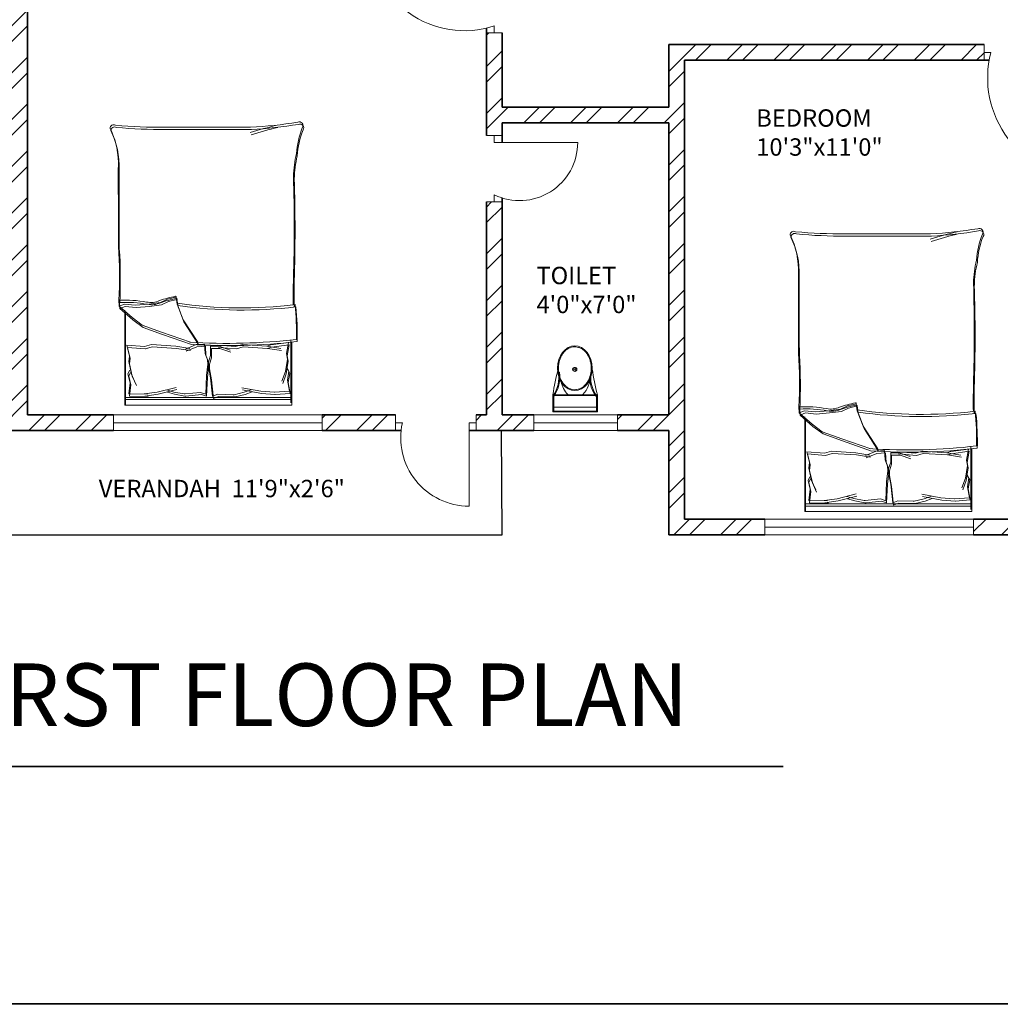
# Model space of a CAD drawing. Units: inches. Extents: x 1885 to 2748, y 783 to 2421.
# Tile 21 of 117: x 2163 to 2445, y 922 to 1206. Entities that reach past the tile are written whole.
import ezdxf

# ---------------------------------------------------------------- set-up
doc = ezdxf.new("R2010")
doc.units = ezdxf.units.IN
for name, color, linetype, lineweight in [('A-ANNO-DIMS', 2, 'Continuous', 18), ('A-ANNO-TTLB', 7, 'Continuous', 35), ('A-AREA-IDEN', 7, 'Continuous', 18), ('A-DOOR', 31, 'Continuous', 18), ('A-FLOR-BALC', 7, 'Continuous', 25), ('A-FLOR-FIXT', 8, 'Continuous', 18), ('A-FURN', 8, 'Continuous', 13), ('A-GLAZ', 181, 'Continuous', 18), ('A-WALL', 7, 'Continuous', 35)]:
    doc.layers.add(name, color=color, linetype=linetype, lineweight=lineweight)
doc.layers.add('A-WALL-PATT', color=85, linetype='Continuous', lineweight=13, true_color=0x58ba48)
doc.styles.get("Standard").update_dxf_attribs({"font": 'arial.ttf'})
doc.dimstyles.get("Standard").update_dxf_attribs({"dimtxt": 0.18, "dimasz": 0.18, "dimexe": 0.18, "dimexo": 0.0625, "dimgap": 0.09, "dimtad": 0, "dimtih": 1, "dimtoh": 1, "dimdec": 4, "dimzin": 0, "dimdsep": 46, "dimtxsty": 'Standard', "dimcen": 0.09, "dimadec": 0, "dimazin": 0, "dimtfac": 1, "dimtdec": 4, "dimtofl": 0, "dimtmove": 0, "dimatfit": 3, "dimfxl": 1, "dimtolj": 1, "dimtzin": 0, "dimarcsym": 0})

# ---------------------------------------------------------------- blocks, each defined once
blk = doc.blocks.new('A$C31115884')
for p, q in [((283, 498), (223, 498)), ((258, 466), (258, 523)), ((0, 200), (0, 0)), ((520, 200), (0, 200)), ((10, 190), (10, 10)), ((510, 190), (10, 190)), ((510, 10), (510, 190)), ((520, 0), (520, 200)), ((510, 54), (0, 54)), ((10, 10), (510, 10)), ((0, 0), (520, 0))]:
    blk.add_line(p, q)
blk.add_circle((256, 496), 23.6)
for centre, radius, start, end in [((2778, -205), 2807, 165.4549, 171.7133), ((-295, 403), 365, 324.2091, 9.3499), ((-295, 403), 375, 324.2091, 9.3499), ((806, 403), 365, 170.6501, 215.7909), ((3237, 905), 2807, 188.2867, 194.5451), ((384, 406), 293, 190.2774, 224.1564), ((139, 406), 293, 315.8436, 2.6563), ((806, 403), 375, 179.2036, 215.7909)]:
    blk.add_arc(centre, radius, start, end)
blk.add_ellipse((256, 510), major_axis=(0, -261), ratio=0.772727)
blk.add_open_spline([(256, 259), (263, 259), (270, 260), (288, 262), (299, 265), (320, 273), (330, 278), (350, 291), (360, 299), (378, 316), (386, 326), (402, 347), (409, 358), (421, 383), (427, 395), (436, 422), (440, 436), (445, 465), (447, 480), (448, 509), (448, 524), (445, 553), (443, 568), (436, 596), (432, 610), (422, 636), (416, 649), (402, 672), (395, 683), (379, 703), (370, 712), (351, 728), (341, 735), (321, 746), (310, 751), (289, 757), (278, 759), (256, 761), (245, 761), (223, 757), (212, 754), (191, 746), (181, 741), (161, 728), (151, 720), (133, 703), (125, 693), (110, 672), (103, 660), (90, 636), (85, 623), (76, 596), (72, 582), (67, 553), (66, 538), (64, 509), (65, 494), (68, 465), (70, 450), (77, 422), (81, 408), (91, 382), (97, 370), (111, 346), (118, 335), (135, 316), (144, 307), (162, 291), (172, 284), (193, 273), (203, 269), (225, 262), (236, 260), (250, 259), (253, 259), (256, 259)], degree=3, knots=[0, 0, 0, 0, 0.110105, 0.110105, 0.285049, 0.285049, 0.459994, 0.459994, 0.634938, 0.634938, 0.809882, 0.809882, 0.984827, 0.984827, 1.159771, 1.159771, 1.334715, 1.334715, 1.50966, 1.50966, 1.684604, 1.684604, 1.859549, 1.859549, 2.034493, 2.034493, 2.209437, 2.209437, 2.384382, 2.384382, 2.559326, 2.559326, 2.73427, 2.73427, 2.909215, 2.909215, 3.084159, 3.084159, 3.259103, 3.259103, 3.434048, 3.434048, 3.608992, 3.608992, 3.783936, 3.783936, 3.958881, 3.958881, 4.133825, 4.133825, 4.30877, 4.30877, 4.483714, 4.483714, 4.658658, 4.658658, 4.833603, 4.833603, 5.008547, 5.008547, 5.183491, 5.183491, 5.358436, 5.358436, 5.53338, 5.53338, 5.708324, 5.708324, 5.883269, 5.883269, 6.058213, 6.058213, 6.233158, 6.233158, 6.283185, 6.283185, 6.283185, 6.283185])
blk = doc.blocks.new('BED-DOUBLE')
for p, q in [((0, 51.49), (0.64, 51.49)), ((0, 3.47), (0, 51.49)), ((0, 51.26), (26.61, 51.26)), ((0, 51.26), (26.61, 51.26)), ((0.64, 51.49), (27.25, 51.49)), ((0.64, 51.49), (27.25, 51.49)), ((1.54, 3.47), (1.54, 51.26)), ((1.54, 3.47), (1.54, 51.26)), ((2.18, 3.7), (2.18, 51.49)), ((2.18, 3.7), (2.18, 51.49)), ((27.75, 52.87), (24.5, 49.16)), ((27.75, 52.87), (24.5, 49.16)), ((28.39, 53.09), (25.14, 49.39)), ((28.39, 53.09), (25.14, 49.39)), ((29.49, 52.95), (27.75, 52.87, 3.87)), ((29.49, 52.95), (27.75, 52.87, 3.87)), ((28.37, 51.33), (27.75, 52.87)), ((28.37, 51.33), (27.75, 52.87)), ((28.06, 48.23), (28.37, 51.33)), ((28.06, 48.23), (28.37, 51.33)), ((30.13, 53.17), (28.39, 53.09, 3.87)), ((30.13, 53.17), (28.39, 53.09, 3.87)), ((29.01, 51.56), (28.39, 53.09)), ((29.01, 51.56), (28.39, 53.09)), ((28.7, 48.46), (29.01, 51.56)), ((28.7, 48.46), (29.01, 51.56)), ((2.56, 50.11), (2.46, 44.71)), ((2.56, 50.11), (2.46, 44.71)), ((2.56, 50.11), (5.77, 49.73)), ((2.56, 50.11), (5.77, 49.73)), ((3.2, 50.34), (3.1, 44.94)), ((3.2, 50.34), (3.1, 44.94)), ((3.2, 50.34), (6.41, 49.96)), ((3.2, 50.34), (6.41, 49.96)), ((8.26, 49.31), (5.58, 48.13)), ((8.26, 49.31), (5.58, 48.13)), ((5.77, 49.73), (8.34, 50.33)), ((5.77, 49.73), (8.34, 50.33)), ((8.9, 49.54), (6.22, 48.36)), ((8.9, 49.54), (6.22, 48.36)), ((6.41, 49.96), (8.98, 50.56)), ((6.41, 49.96), (8.98, 50.56)), ((11.83, 50.11), (8.26, 49.31)), ((11.83, 50.11), (8.26, 49.31)), ((8.34, 50.33), (9.39, 49.81)), ((8.34, 50.33), (9.39, 49.81)), ((12.47, 50.34), (8.9, 49.54)), ((12.47, 50.34), (8.9, 49.54)), ((8.98, 50.56), (10.03, 50.04)), ((8.98, 50.56), (10.03, 50.04)), ((13.44, 49.92), (11.83, 50.11)), ((13.44, 49.92), (11.83, 50.11)), ((14.08, 50.15), (12.47, 50.34)), ((14.08, 50.15), (12.47, 50.34)), ((16.58, 50.7), (13.44, 49.92)), ((16.58, 50.7), (13.44, 49.92)), ((17.22, 50.93), (14.08, 50.15)), ((17.22, 50.93), (14.08, 50.15)), ((16.17, 45.57), (16.58, 50.7)), ((16.17, 45.56), (16.58, 50.7)), ((16.81, 45.79), (17.22, 50.93)), ((16.81, 45.79), (17.22, 50.93)), ((24.5, 49.16), (22.33, 46.22)), ((24.5, 49.16), (22.33, 46.22)), ((25.14, 49.39), (22.97, 46.45)), ((25.14, 49.39), (22.97, 46.45)), ((28.37, 44.36), (28.06, 48.23)), ((28.37, 44.36), (28.06, 48.23)), ((29.01, 44.59), (28.7, 48.46)), ((29.01, 44.59), (28.7, 48.46)), ((2.46, 44.71), (2.55, 45.71)), ((2.46, 44.71), (2.55, 45.71)), ((2.55, 45.71), (3.07, 41.91)), ((2.55, 45.71), (3.07, 41.91)), ((3.1, 44.94), (3.19, 45.94)), ((3.1, 44.94), (3.19, 45.94)), ((3.19, 45.94), (3.71, 42.14)), ((3.19, 45.94), (3.71, 42.14)), ((16.73, 43.6), (16.17, 45.57)), ((16.73, 43.6), (16.17, 45.56)), ((17.37, 43.83), (16.81, 45.79)), ((17.37, 43.83), (16.81, 45.79)), ((22.33, 46.22), (20.32, 40.64)), ((22.33, 46.22), (20.32, 40.64)), ((22.97, 46.45), (20.96, 40.87)), ((22.97, 46.45), (20.96, 40.87)), ((16.3, 36.59), (16.73, 43.6)), ((16.3, 36.59), (16.73, 43.6)), ((16.94, 36.82), (17.37, 43.83)), ((16.94, 36.82), (17.37, 43.83)), ((28.83, 40.95), (28.37, 44.36)), ((28.83, 40.95), (28.37, 44.36)), ((29.47, 41.18), (29.01, 44.59)), ((29.47, 41.18), (29.01, 44.59)), ((3.07, 41.91), (4.43, 36.49)), ((3.07, 41.91), (4.43, 36.49)), ((3.71, 42.14), (5.07, 36.72)), ((3.71, 42.14), (5.07, 36.72)), ((20.32, 40.64), (17.39, 32.3)), ((20.32, 40.64), (17.39, 32.3)), ((20.96, 40.87), (18.03, 32.53)), ((20.96, 40.87), (18.03, 32.53)), ((29.76, 38.94), (28.83, 40.95)), ((29.76, 38.94), (28.83, 40.95)), ((30.4, 39.17), (29.47, 41.18)), ((30.4, 39.17), (29.47, 41.18)), ((79.25, 15.06), (79.25, 39.68)), ((79.25, 15.06), (79.25, 39.68)), ((79.89, 15.29), (79.89, 39.9)), ((79.89, 15.29), (79.89, 39.9)), ((3.08, 37.13), (2.54, 34.2)), ((3.08, 37.13), (2.54, 34.2)), ((3.68, 39.2), (3.08, 37.13)), ((3.68, 39.2), (3.08, 37.13)), ((3.72, 37.36), (3.18, 34.43)), ((3.72, 37.36), (3.18, 34.43)), ((4.32, 39.43), (3.72, 37.36)), ((4.32, 39.43), (3.72, 37.36)), ((16.27, 32.79), (16.94, 36.82)), ((16.27, 32.79), (16.94, 36.82)), ((30.38, 36.46), (29.76, 38.94)), ((30.38, 36.46), (29.76, 38.94)), ((31.02, 36.69), (30.4, 39.17)), ((31.02, 36.69), (30.4, 39.17)), ((2.54, 34.2), (2.56, 33.88)), ((2.54, 34.2), (2.56, 33.88)), ((3.18, 34.43), (3.2, 34.11)), ((3.18, 34.43), (3.2, 34.11)), ((3.2, 34.11), (3.62, 29.68)), ((3.2, 34.11), (3.62, 29.68)), ((15.63, 32.56), (16.3, 36.59)), ((15.63, 32.56), (16.3, 36.59)), ((17.38, 30.98), (16.1, 34.05)), ((17.38, 30.98), (16.1, 34.05)), ((17.39, 30.26), (23.88, 34.45)), ((17.39, 30.26), (23.88, 34.45)), ((18.03, 30.49), (24.52, 34.68)), ((18.03, 30.49), (24.52, 34.68)), ((23.88, 34.45), (28.37, 36.15)), ((23.88, 34.45), (28.37, 36.15)), ((24.52, 34.68), (29.01, 36.38)), ((24.52, 34.68), (29.01, 36.38)), ((28.37, 36.15), (30.38, 36.46)), ((28.37, 36.15), (30.38, 36.46)), ((29.01, 36.38), (31.02, 36.69)), ((29.01, 36.38), (31.02, 36.69)), ((2.56, 33.88), (2.98, 29.45)), ((2.56, 33.88), (2.98, 29.45)), ((16.74, 30.75), (15.46, 33.82)), ((16.74, 30.75), (15.46, 33.82)), ((2.98, 29.45), (2.5, 27.98)), ((2.98, 29.45), (2.5, 27.98)), ((3.62, 29.68), (3.13, 28.2)), ((3.62, 29.68), (3.13, 28.2)), ((13.02, 27.66), (14.86, 28.36)), ((13.02, 27.66), (14.86, 28.36)), ((14.86, 28.36), (17.54, 28.52)), ((14.86, 28.36), (17.54, 28.52)), ((16.9, 28.3), (16.74, 30.75)), ((16.9, 28.3), (16.74, 30.75)), ((17.54, 28.52), (17.38, 30.98)), ((17.54, 28.52), (17.38, 30.98)), ((1.87, 25.98), (7.22, 26.56)), ((1.87, 25.98), (7.22, 26.56)), ((2.45, 24.54), (1.87, 25.98)), ((2.45, 24.54), (1.87, 25.98)), ((2.5, 27.98), (7.87, 27.73)), ((2.5, 27.98), (7.87, 27.73)), ((2.51, 26.21), (7.86, 26.79)), ((2.51, 26.21), (7.86, 26.79)), ((3.09, 24.76), (2.51, 26.21)), ((3.09, 24.76), (2.51, 26.21)), ((3.13, 28.2), (8.51, 27.96)), ((3.13, 28.2), (8.51, 27.96)), ((7.22, 26.56), (10.4, 27.14)), ((7.22, 26.56), (10.4, 27.14)), ((7.86, 26.79), (11.04, 27.37)), ((7.86, 26.79), (11.04, 27.37)), ((7.87, 27.73), (11.08, 27.35)), ((7.87, 27.73), (11.08, 27.35)), ((8.51, 27.96), (11.72, 27.58)), ((8.51, 27.96), (11.72, 27.58)), ((10.4, 27.14), (11.71, 27.14)), ((10.4, 27.14), (11.71, 27.14)), ((11.04, 27.37), (12.35, 27.37)), ((11.04, 27.37), (12.35, 27.37)), ((11.08, 27.35), (12.38, 27.43)), ((11.08, 27.35), (12.38, 27.43)), ((11.71, 27.14), (13.59, 26.56)), ((11.71, 27.14), (13.59, 26.56)), ((11.72, 27.58), (13.02, 27.66)), ((11.72, 27.58), (13.02, 27.66)), ((12.35, 27.37), (14.22, 26.79)), ((12.35, 27.37), (14.22, 26.79)), ((12.38, 27.43), (14.22, 28.13)), ((12.38, 27.43), (14.22, 28.13)), ((13.59, 26.56), (16.27, 26.56)), ((13.59, 26.56), (16.27, 26.56)), ((14.22, 28.13), (16.9, 28.3)), ((14.22, 28.13), (16.9, 28.3)), ((14.22, 26.79), (16.91, 26.79)), ((14.22, 26.79), (16.91, 26.79)), ((16.27, 26.56), (16.27, 24.1)), ((16.27, 26.56), (16.27, 24.1)), ((16.91, 26.79), (16.91, 24.33)), ((16.91, 26.79), (16.91, 24.33)), ((2.31, 20.09), (2.45, 24.54)), ((2.31, 20.09), (2.45, 24.54)), ((2.95, 20.32), (3.09, 24.76)), ((2.95, 20.32), (3.09, 24.76)), ((16.27, 24.1), (15.18, 20.96)), ((16.27, 24.1), (15.18, 20.96)), ((16.91, 24.33), (15.82, 21.19)), ((16.91, 24.33), (15.82, 21.19)), ((16.17, 19.38), (16.58, 24.51)), ((16.17, 19.38), (16.58, 24.51)), ((16.81, 19.61), (17.22, 24.74)), ((16.81, 19.61), (17.22, 24.74)), ((2.31, 19.77), (2.31, 20.09)), ((2.31, 19.77), (2.31, 20.09)), ((2.95, 20), (2.95, 20.32)), ((2.95, 20), (2.95, 20.32)), ((3.67, 17.11), (2.95, 20)), ((3.67, 17.11), (2.95, 20)), ((3.03, 16.88), (2.31, 19.77)), ((3.03, 16.88), (2.31, 19.77)), ((3.32, 12.11), (4.33, 17.6)), ((3.32, 12.11), (4.33, 17.6)), ((4.39, 15.08), (3.67, 17.11)), ((4.39, 15.08), (3.67, 17.11)), ((3.96, 12.34), (4.97, 17.83)), ((3.96, 12.34), (4.97, 17.83)), ((16.73, 17.42), (16.17, 19.38)), ((16.73, 17.42), (16.17, 19.38)), ((16.3, 10.41), (16.73, 17.42)), ((16.3, 10.41), (16.73, 17.42)), ((17.37, 17.65), (16.81, 19.61)), ((17.37, 17.65), (16.81, 19.61)), ((16.94, 10.64), (17.37, 17.65)), ((16.94, 10.64), (17.37, 17.65)), ((3.75, 14.85), (3.03, 16.88)), ((3.75, 14.85), (3.03, 16.88)), ((3.03, 8.28), (3.32, 12.11)), ((3.03, 8.28), (3.32, 12.11)), ((3.67, 8.51), (3.96, 12.34)), ((3.67, 8.51), (3.96, 12.34)), ((3.65, 8.41), (3.67, 8.51)), ((3.65, 8.41), (3.67, 8.51)), ((15.63, 6.38), (16.3, 10.41)), ((15.63, 6.38), (16.3, 10.41)), ((16.27, 6.61), (16.94, 10.64)), ((16.27, 6.61), (16.94, 10.64)), ((16.3, 10.41), (16.62, 9.28)), ((16.3, 10.41), (16.62, 9.28)), ((16.62, 9.28), (17.34, 4.18)), ((16.62, 9.28), (17.34, 4.18)), ((16.94, 10.64), (17.26, 9.51)), ((16.94, 10.64), (17.26, 9.51)), ((17.26, 9.51), (17.98, 4.41)), ((17.26, 9.51), (17.98, 4.41)), ((3.01, 8.18), (3.03, 8.28)), ((3.01, 8.18), (3.03, 8.28)), ((3.34, 3.9), (3.01, 8.18)), ((3.34, 3.9), (3.01, 8.18)), ((3.98, 4.13), (3.65, 8.41)), ((3.98, 4.13), (3.65, 8.41)), ((8.96, 5.05), (6.21, 6.06)), ((8.96, 5.05), (6.21, 6.06)), ((9.6, 5.28), (6.85, 6.29)), ((9.6, 5.28), (6.85, 6.29)), ((18.11, 3.47), (0, 3.47)), ((18.11, 3.47), (0, 3.47)), ((18.75, 3.7), (0.64, 3.7)), ((18.75, 3.7), (0.64, 3.7)), ((3.32, 3.89), (6.5, 4.47)), ((3.32, 3.89), (6.5, 4.47)), ((3.96, 4.12), (7.14, 4.7)), ((3.96, 4.12), (7.14, 4.7)), ((6.5, 4.47), (9.1, 4.04)), ((6.5, 4.47), (9.1, 4.04)), ((7.14, 4.7), (9.74, 4.27)), ((7.14, 4.7), (9.74, 4.27)), ((12.57, 4.47), (8.96, 5.05)), ((12.57, 4.47), (8.96, 5.05)), ((9.1, 4.04), (10.12, 4.62)), ((9.1, 4.04), (10.12, 4.62)), ((13.21, 4.7), (9.6, 5.28)), ((13.21, 4.7), (9.6, 5.28)), ((9.74, 4.27), (10.75, 4.84)), ((9.74, 4.27), (10.75, 4.84)), ((14.16, 4.76), (12.57, 4.47)), ((14.16, 4.76), (12.57, 4.47)), ((14.8, 4.99), (13.21, 4.7)), ((14.8, 4.99), (13.21, 4.7)), ((17.34, 4.18), (14.16, 4.76)), ((17.34, 4.18), (14.16, 4.76)), ((17.98, 4.41), (14.8, 4.99)), ((17.98, 4.41), (14.8, 4.99))]:
    blk.add_line(p, q)
for centre, radius, start, end in [((68.67, 76.16), 23.07, 267.4714, 296.4681), ((68.67, 76.16), 23.07, 267.4714, 296.4681), ((69.31, 76.38), 23.07, 267.4714, 296.4681), ((69.31, 76.38), 23.07, 267.4714, 296.4681), ((78.87, 54.41), 1.1, 332.6588, 86.02), ((78.87, 54.41), 1.1, 332.6588, 86.02), ((212.28, 41.15), 133.04, 174.4998, 180.6351), ((212.28, 41.15), 133.04, 174.4998, 180.6351), ((79.51, 54.64), 1.1, 332.6588, 86.02), ((79.51, 54.64), 1.1, 332.6588, 86.02), ((212.92, 41.38), 133.04, 174.4998, 180.6351), ((212.92, 41.38), 133.04, 174.4998, 180.6351), ((-6.65, 51.33), 36.18, 349.8763, 2.5657), ((-6.65, 51.33), 36.18, 349.8763, 2.5657), ((36.32, 182.26), 129.5, 266.9791, 273.8365), ((36.32, 182.26), 129.5, 266.9791, 273.8365), ((-6.01, 51.55), 36.18, 349.8763, 2.5657), ((-6.01, 51.55), 36.18, 349.8763, 2.5657), ((36.96, 182.49), 129.5, 266.9791, 273.8365), ((36.96, 182.49), 129.5, 266.9791, 273.8365), ((67.83, -4508.74), 4561.86, 90.00217, 90.28689), ((67.83, -4508.75), 4561.86, 90.00217, 90.28689), ((68.46, -4508.52), 4561.86, 90.00217, 90.28689), ((68.46, -4508.52), 4561.86, 90.00217, 90.28689), ((35.07, 43.74), 6.22, 168.6608, 203.7384), ((35.07, 43.74), 6.22, 168.6608, 203.7384), ((35.71, 43.97), 6.22, 168.6608, 203.7384), ((35.71, 43.97), 6.22, 168.6608, 203.7384), ((1.49, 31.15), 29.65, 10.6617, 19.8806), ((1.49, 31.15), 29.65, 10.6617, 19.8806), ((2.13, 31.38), 29.65, 10.6617, 19.8806), ((2.13, 31.38), 29.65, 10.6617, 19.8806), ((31.08, 36.86), 0.185, 250.2464, 1.1377), ((31.08, 36.86), 0.185, 250.2464, 1.1377), ((156.32, 17.75), 129.02, 171.7845, 186.9006), ((156.32, 17.75), 129.02, 171.7845, 186.9006), ((156.96, 17.98), 129.02, 171.7845, 186.9006), ((156.96, 17.98), 129.02, 171.7845, 186.9006), ((30.44, 36.64), 0.185, 250.2464, 1.1377), ((30.44, 36.63), 0.185, 250.2464, 1.1377), ((182.06, 21.36), 164.97, 176.0865, 186.7821), ((182.06, 21.36), 164.97, 176.0865, 186.7821), ((182.7, 21.59), 164.97, 176.0865, 186.7821), ((182.7, 21.59), 164.97, 176.0865, 186.7821), ((-23.71, -17.22), 106.46, 13.3832, 17.7053), ((-23.71, -17.22), 106.46, 13.3832, 17.7053), ((-23.07, -16.99), 106.46, 13.3832, 17.7053), ((-23.07, -16.99), 106.46, 13.3832, 17.7053), ((200.84, 21.43), 121.76, 182.9958, 189.4091), ((200.84, 21.43), 121.76, 182.9958, 189.4091), ((201.48, 21.65), 121.76, 182.9958, 189.4091), ((201.48, 21.65), 121.76, 182.9958, 189.4091), ((31.82, -167.08), 170.11, 88.4762, 91.0082), ((31.82, -167.08), 170.11, 88.4762, 91.0082), ((51.26, 485.05), 482.31, 268.2277, 271.7185), ((51.26, 485.05), 482.31, 268.2277, 271.7185), ((65.16, -26.67), 29.63, 76.0648, 88.9113), ((65.16, -26.67), 29.63, 76.0648, 88.9113), ((20.1, 85.16), 83.31, 268.7218, 275.604), ((20.1, 85.16), 83.31, 268.7218, 275.604), ((20.74, 85.39), 83.31, 268.7218, 275.604), ((20.74, 85.39), 83.31, 268.7218, 275.604), ((31.18, -167.31), 170.11, 88.4762, 91.0082), ((31.18, -167.31), 170.11, 88.4762, 91.0082), ((50.62, 484.82), 482.31, 268.2277, 271.7185), ((50.62, 484.82), 482.31, 268.2277, 271.7185), ((64.52, -26.9), 29.63, 76.0648, 88.9113), ((64.52, -26.9), 29.63, 76.0648, 88.9113), ((70.28, -21.66), 23.56, 67.9751, 86.652), ((70.28, -21.66), 23.56, 67.9751, 86.652), ((70.92, -21.43), 23.56, 67.9751, 86.652), ((70.92, -21.43), 23.56, 67.9751, 86.652), ((79.72, 1.09), 1.09, 236.1736, 23.4781), ((79.72, 1.09), 1.09, 236.1736, 23.4781), ((80.36, 1.31), 1.09, 236.1736, 23.4781), ((80.36, 1.31), 1.09, 236.1736, 23.4781)]:
    blk.add_arc(centre, radius, start, end)
blk = doc.blocks.new('WIN-60')
for p, q in [((0, 60), (4.5, 60)), ((0, 60), (0, 0)), ((4.5, 60), (2.25, 60)), ((2.25, 60), (2.25, 0)), ((4.5, 0), (4.5, 60)), ((2.25, 0), (0, 0)), ((0, 0), (4.5, 0))]:
    blk.add_line(p, q)
blk = doc.blocks.new('WIN-24')
for p, q in [((0, 4.5), (0, 0)), ((0, 4.5), (24, 4.5)), ((24, 2.25), (24, 4.5)), ((24, 4.5), (24, 0)), ((0, 0), (0, 2.25)), ((0, 2.25), (24, 2.25)), ((24, 0), (0, 0))]:
    blk.add_line(p, q)
blk = doc.blocks.new('*D43')
at = {"layer": 'A-ANNO-DIMS', "color": 0, "lineweight": -2, "transparency": 16777216}
for p, q in [((1971.27, 1057.44), (1971.27, 922.48)), ((2618.27, 1057.44), (2618.27, 922.48)), ((1971.45, 922.66), (2294.48, 922.66)), ((2618.09, 922.66), (2295.06, 922.66))]:
    blk.add_line(p, q, dxfattribs=at)
at = {"layer": 'A-ANNO-DIMS', "color": 0, "transparency": 16777216}
for points in [[(1971.45, 922.69), (1971.45, 922.63), (1971.27, 922.66)], [(2618.09, 922.69), (2618.09, 922.63), (2618.27, 922.66)]]:
    blk.add_solid(points, dxfattribs=at)
at = {"layer": 'Defpoints', "color": 0, "transparency": 16777216}
for p in [(1971.27, 1057.51), (2618.27, 1057.51), (2618.27, 922.66)]:
    blk.add_point(p, dxfattribs=at)
at = {"layer": 'A-ANNO-DIMS', "color": 0, "transparency": 16777216, "insert": (2294.77, 922.66), "char_height": 0.18, "attachment_point": 5}
blk.add_mtext('\\A1;647', dxfattribs=at)

msp = doc.modelspace()

# ---------------------------------------------------------------- hatches: boundary and pattern name
at = {"layer": 'A-WALL-PATT'}
h = msp.add_hatch(dxfattribs=at)
h.set_pattern_fill('ANSI32', color=256)
h.paths.add_polyline_path([(2007.77, 2318.01), (1980.77, 2318.01), (1980.77, 2281.22), (1985.27, 2281.22), (1985.27, 2313.51), (2007.77, 2313.51), (2007.77, 2315.76)])
h.paths.add_polyline_path([(2094.32, 2318.01), (2067.77, 2318.01), (2067.77, 2313.51), (2094.32, 2313.51), (2094.32, 2315.76)])
h.paths.add_polyline_path([(2131.37, 2315.76), (2131.37, 2318.01), (2131.19, 2318.01), (2112.61, 2318.01), (2112.61, 2313.51), (2117.27, 2313.51), (2117.27, 2255.2), (2121.77, 2255.2), (2121.77, 2313.51), (2131.37, 2313.51)])
h.paths.add_polyline_path([(2190.51, 2318.01), (2155.37, 2318.01), (2155.37, 2313.51), (2169.77, 2313.51), (2169.77, 2229.51), (2121.77, 2229.51), (2121.77, 2233.45), (2119.52, 2233.45), (2117.27, 2233.45), (2117.27, 2201.1), (2121.77, 2201.1), (2121.77, 2225.01), (2169.77, 2225.01), (2169.77, 2165.01), (2306.27, 2165.01), (2306.27, 2066.01), (2310.77, 2066.01), (2344.27, 2066.01), (2486.27, 2066.01), (2486.27, 1886.01), (2483.02, 1886.01), (2483.02, 1881.51), (2486.27, 1881.51), (2486.27, 1880.68), (2490.77, 1880.68), (2490.77, 2070.51), (2344.27, 2070.51), (2310.77, 2070.51), (2310.77, 2165.01), (2310.77, 2173.64), (2308.52, 2173.64), (2306.27, 2173.64), (2306.27, 2169.51), (2174.27, 2169.51), (2174.27, 2313.51), (2190.51, 2313.51), (2190.51, 2315.76)])
h.paths.add_polyline_path([(1985.27, 2221.22), (1980.77, 2221.22), (1980.77, 2165.01), (1992.77, 2165.01), (1992.77, 2141.93), (1997.27, 2141.93), (1997.27, 2165.01), (2117.27, 2165.01), (2117.27, 2163.13), (2121.77, 2163.13), (2121.77, 2172.73), (2119.52, 2172.73), (2117.27, 2172.73), (2117.27, 2169.51), (1985.27, 2169.51)])
h.paths.add_polyline_path([(1997.27, 2105.93), (1992.77, 2105.93), (1992.77, 2070.51), (2016.77, 2070.51), (2016.77, 2059.12), (2019.02, 2059.12), (2021.27, 2059.12), (2021.27, 2070.51), (2117.27, 2070.51), (2117.27, 2022.51), (2114.42, 2022.51), (2114.42, 2018.01), (2123.63, 2018.01), (2123.63, 2020.26), (2123.63, 2022.51), (2121.77, 2022.51), (2121.77, 2142.59), (2119.52, 2142.59), (2117.27, 2142.59), (2117.27, 2075.01), (1997.27, 2075.01)])
h.paths.add_polyline_path([(2092.03, 2020.26), (2092.03, 2022.51), (2021.27, 2022.51), (2021.27, 2035.12), (2016.77, 2035.12), (2016.77, 2018.01), (2016.77, 1978.78), (2021.27, 1978.78), (2021.27, 2018.01), (2092.03, 2018.01)])
h.paths.add_polyline_path([(2260.94, 2022.51), (2153.1, 2022.51), (2153.1, 2020.26), (2153.1, 2018.01), (2155.27, 2018.01), (2155.27, 1886.01), (2107.63, 1886.01), (2107.63, 1881.51), (2182.91, 1881.51), (2182.91, 1883.76), (2182.91, 1886.01), (2159.77, 1886.01), (2159.77, 2018.01), (2260.94, 2018.01), (2260.94, 2020.26)])
h.paths.add_polyline_path([(2047.63, 1883.76), (2047.63, 1886.01), (2021.27, 1886.01), (2021.27, 1918.78), (2019.02, 1918.78), (2016.77, 1918.78), (2016.77, 1881.51), (2047.63, 1881.51)])
h.paths.add_polyline_path([(2306.36, 1883.76), (2306.36, 1886.01), (2296.27, 1886.01), (2296.27, 1982.01), (2316.54, 1982.01), (2316.54, 1984.26), (2316.54, 1986.51), (2296.27, 1986.51), (2296.27, 2022.51), (2289.28, 2022.51), (2289.28, 2018.01), (2291.77, 2018.01), (2291.77, 1886.01), (2242.91, 1886.01), (2242.91, 1881.51), (2306.36, 1881.51)], flags=17)
h.paths.add_polyline_path([(1985.27, 1843.01), (2021.6, 1843.01), (2021.53, 1845.44), (2021.48, 1847.51), (1980.77, 1847.51), (1980.77, 1809.45), (1985.27, 1809.45)])
h.paths.add_polyline_path([(2131.48, 1845.26), (2131.48, 1847.51), (2081.53, 1847.51), (2081.53, 1843.01), (2117.27, 1843.01), (2117.27, 1784.15), (2119.52, 1784.15), (2121.77, 1784.15), (2121.77, 1843.01), (2131.48, 1843.01)])
h.paths.add_polyline_path([(2203.89, 1847.51), (2155.48, 1847.51), (2155.48, 1843.01), (2169.77, 1843.01), (2169.77, 1759.01), (2121.77, 1759.01), (2121.77, 1761.46), (2117.27, 1761.46), (2117.27, 1730.43), (2121.77, 1730.43), (2121.77, 1754.51), (2177.42, 1754.51), (2177.42, 1756.76), (2177.42, 1759.01), (2174.27, 1759.01), (2174.27, 1843.01), (2203.89, 1843.01)])
h.paths.add_polyline_path([(2335.55, 1845.26), (2335.55, 1847.51), (2239.89, 1847.51), (2239.89, 1843.01), (2306.27, 1843.01), (2306.27, 1759.01), (2199.49, 1759.01), (2199.49, 1754.51), (2310.77, 1754.51), (2310.77, 1843.01), (2335.55, 1843.01)])
h.paths.add_polyline_path([(2348.77, 2022.51), (2344.27, 2022.51), (2344.27, 1986.51), (2341.68, 1986.51), (2341.68, 1982.01), (2344.27, 1982.01), (2344.27, 1886.01), (2330.36, 1886.01), (2330.36, 1881.51), (2361.63, 1881.51), (2361.63, 1883.76), (2361.63, 1886.01), (2348.77, 1886.01)], flags=17)
h.paths.add_polyline_path([(2283.25, 2315.76), (2283.25, 2318.01), (2238.51, 2318.01), (2238.51, 2313.51), (2283.25, 2313.51)], flags=17)
h.paths.add_polyline_path([(2363.27, 2348.01), (2388.68, 2348.01), (2388.68, 2350.26), (2388.68, 2352.51), (2358.77, 2352.51), (2358.77, 2348.01), (2358.77, 2318.01), (2344.48, 2318.01), (2344.48, 2313.51), (2358.77, 2313.51), (2358.77, 2229.51), (2310.77, 2229.51), (2310.77, 2231.95), (2306.27, 2231.95), (2306.27, 2205.61), (2310.77, 2205.61), (2310.77, 2225.01), (2358.77, 2225.01), (2358.77, 2211.51), (2452.33, 2211.51), (2452.33, 2213.76), (2452.33, 2216.01), (2363.27, 2216.01), (2363.27, 2318.01)])
h.paths.add_polyline_path([(2310.77, 2313.51), (2320.48, 2313.51), (2320.48, 2315.76), (2320.48, 2318.01), (2302.73, 2318.01), (2302.73, 2313.51), (2306.27, 2313.51), (2306.27, 2251.08), (2310.77, 2251.08)], flags=17)
h.paths.add_polyline_path([(2490.77, 2352.51), (2486.27, 2352.51), (2448.68, 2352.51), (2448.68, 2348.01), (2486.27, 2348.01), (2486.27, 2318.01), (2486.27, 2216.01), (2481.78, 2216.01), (2481.78, 2211.51), (2486.27, 2211.51), (2486.27, 2165.01), (2493.29, 2165.01), (2493.29, 2167.26), (2493.29, 2169.51), (2490.77, 2169.51), (2490.77, 2313.51), (2494.43, 2313.51), (2494.43, 2318.01), (2490.77, 2318.01)])
h.paths.add_polyline_path([(2534.65, 2318.01), (2515.69, 2318.01), (2515.69, 2313.51), (2534.65, 2313.51), (2534.65, 2315.76)])
h.paths.add_polyline_path([(2618.27, 2318.01), (2594.65, 2318.01), (2594.65, 2313.51), (2613.77, 2313.51), (2613.77, 2281.71), (2618.27, 2281.71)])
h.paths.add_polyline_path([(2618.27, 2221.71), (2613.77, 2221.71), (2613.77, 2169.51), (2554.02, 2169.51), (2554.02, 2165.01), (2613.77, 2165.01), (2613.77, 2152.88), (2618.27, 2152.88)])
h.paths.add_polyline_path([(2618.27, 2128.88), (2616.02, 2128.88), (2613.77, 2128.88), (2613.77, 2117.01), (2529.77, 2117.01), (2529.77, 2165.01), (2532.85, 2165.01), (2532.85, 2169.51), (2522.87, 2169.51), (2522.87, 2165.01), (2525.27, 2165.01), (2525.27, 2117.01), (2525.27, 2112.51), (2525.27, 2108.58), (2529.77, 2108.58), (2529.77, 2112.51), (2613.77, 2112.51), (2613.77, 2080.19), (2618.27, 2080.19)])
h.paths.add_polyline_path([(2618.27, 2044.19), (2616.02, 2044.19), (2613.77, 2044.19), (2613.77, 2015.51), (2529.77, 2015.51), (2529.77, 2088.58), (2527.52, 2088.58), (2525.27, 2088.58), (2525.27, 2011.01), (2613.77, 2011.01), (2613.77, 1956.75), (2618.27, 1956.75)])
h.paths.add_polyline_path([(2618.27, 1881.51), (2618.27, 1896.75), (2613.77, 1896.75), (2613.77, 1881.51), (2613.77, 1847.51), (2592.71, 1847.51), (2592.71, 1843.01), (2613.77, 1843.01), (2613.77, 1765.01), (2613.77, 1760.51), (2609.62, 1760.51), (2609.62, 1756.01), (2613.77, 1756.01), (2613.77, 1660.01), (2608.54, 1660.01), (2608.54, 1655.51), (2613.77, 1655.51), (2613.77, 1508.16), (2618.27, 1508.16)])
h.paths.add_polyline_path([(2565.77, 1843.01), (2569, 1843.01), (2569, 1847.51), (2490.77, 1847.51), (2490.77, 1849.7), (2488.52, 1849.7), (2486.27, 1849.7), (2486.27, 1847.51), (2477.27, 1847.51), (2477.27, 1838.51), (2477.27, 1821.49), (2486.27, 1821.49), (2486.27, 1838.51), (2561.27, 1838.51), (2561.27, 1765.01), (2486.27, 1765.01), (2486.27, 1786.16), (2477.27, 1786.16), (2477.27, 1765.01), (2477.27, 1756.01), (2486.27, 1756.01), (2565.77, 1756.01), (2585.62, 1756.01), (2585.62, 1758.26), (2585.62, 1760.51), (2565.77, 1760.51), (2565.77, 1765.01)])
h.paths.add_polyline_path([(2486.27, 1651.01), (2561.27, 1651.01), (2561.27, 1567.01), (2486.27, 1567.01), (2486.27, 1591.32), (2477.27, 1591.32), (2477.27, 1567.01), (2477.27, 1558.01), (2477.27, 1555.44), (2481.77, 1555.44), (2481.77, 1558.01), (2568.65, 1558.01), (2568.65, 1560.26), (2568.65, 1562.51), (2565.77, 1562.51), (2565.77, 1655.51), (2584.54, 1655.51), (2584.54, 1657.76), (2584.54, 1660.01), (2565.77, 1660.01), (2486.27, 1660.01), (2477.27, 1660.01), (2477.27, 1651.01), (2477.27, 1632.99), (2486.27, 1632.99)])
h.paths.add_polyline_path([(2449.97, 1883.76), (2449.97, 1886.01), (2421.63, 1886.01), (2421.63, 1881.51), (2449.97, 1881.51)], flags=17)
h.paths.add_polyline_path([(2447.27, 1847.51), (2395.55, 1847.51), (2395.55, 1843.01), (2442.77, 1843.01), (2442.77, 1809.27), (2447.27, 1809.27)])
h.paths.add_polyline_path([(1985.27, 1749.45), (1980.77, 1749.45), (1980.77, 1694.5), (1985.27, 1694.5), (1985.27, 1694.51), (1986.9, 1694.51), (1986.9, 1697.78), (1986.9, 1699.01), (1985.27, 1699.01)])
h.paths.add_polyline_path([(2152.77, 1699.01), (2121.77, 1699.01), (2121.77, 1703.67), (2119.52, 1703.67), (2117.27, 1703.67), (2117.27, 1699.01), (2009.22, 1699.01), (2009.22, 1694.51), (2148.27, 1694.51), (2148.27, 1692.63), (2152.77, 1692.63)])
h.paths.add_polyline_path([(2016.27, 1694.51), (2011.77, 1694.51), (2011.77, 1558.01), (2040.81, 1558.01), (2040.81, 1560.26), (2040.81, 1562.51), (2016.27, 1562.51)])
h.paths.add_polyline_path([(2152.77, 1663.02), (2150.52, 1663.02), (2148.27, 1663.02), (2148.27, 1562.51), (2100.81, 1562.51), (2100.81, 1558.01), (2165.12, 1558.01), (2165.12, 1560.26), (2165.12, 1562.51), (2152.77, 1562.51), (2152.77, 1610.51), (2224.77, 1610.51), (2224.77, 1607.99), (2229.27, 1607.99), (2229.27, 1615.01), (2152.77, 1615.01)])
h.paths.add_polyline_path([(2238.61, 1560.26), (2238.61, 1562.51), (2229.27, 1562.51), (2229.27, 1588.76), (2227.02, 1588.76), (2224.77, 1588.77), (2224.77, 1562.51), (2189.12, 1562.51), (2189.12, 1558.01), (2238.61, 1558.01)])
h.paths.add_polyline_path([(2336.02, 1560.26), (2336.02, 1562.51), (2310.77, 1562.51), (2310.77, 1656.35), (2308.52, 1656.35), (2306.27, 1656.35), (2306.27, 1562.51), (2286.61, 1562.51), (2286.61, 1558.01), (2336.02, 1558.01)])
h.paths.add_polyline_path([(2447.27, 1690.97), (2445.02, 1690.97), (2442.77, 1690.97), (2442.77, 1687.01), (2306.27, 1687.01), (2306.27, 1680.75), (2310.77, 1680.75), (2310.77, 1682.51), (2442.77, 1682.51), (2442.77, 1562.51), (2396.02, 1562.51), (2396.02, 1558.01), (2447.27, 1558.01)])
h.paths.add_polyline_path([(2447.27, 1749.27), (2445.02, 1749.27), (2442.77, 1749.27), (2442.77, 1717.23), (2447.27, 1717.23)])
h.paths.add_polyline_path([(2044.67, 1521.76), (2044.67, 1524.01), (2007.27, 1524.01), (2007.27, 1503.49), (2009.52, 1503.49), (2011.77, 1503.49), (2011.77, 1519.51), (2044.67, 1519.51)])
h.paths.add_polyline_path([(2177.97, 1521.76), (2177.97, 1524.01), (2104.67, 1524.01), (2104.67, 1519.51), (2145.77, 1519.51), (2145.77, 1387.51), (2143.37, 1387.51), (2143.37, 1383.01), (2251.59, 1383.01), (2251.59, 1385.26), (2251.59, 1387.51), (2150.27, 1387.51), (2150.27, 1519.51), (2177.97, 1519.51)])
h.paths.add_polyline_path([(2298.7, 1524.01), (2237.97, 1524.01), (2237.97, 1519.51), (2282.27, 1519.51), (2282.27, 1387.51), (2279.68, 1387.51), (2279.68, 1383.01), (2286.77, 1383.01), (2286.77, 1419.01), (2312.45, 1419.01), (2312.45, 1421.26), (2312.45, 1423.51), (2286.77, 1423.51), (2286.77, 1519.51), (2298.7, 1519.51), (2298.7, 1521.72)], flags=17)
h.paths.add_polyline_path([(2361.9, 1521.76), (2361.9, 1524.01), (2322.7, 1524.01), (2322.7, 1519.51), (2334.77, 1519.51), (2334.77, 1423.51), (2331.93, 1423.51), (2331.93, 1419.01), (2334.77, 1419.01), (2334.77, 1387.51), (2334.77, 1383.23), (2339.27, 1383.23), (2339.27, 1387.51), (2339.27, 1519.51), (2361.9, 1519.51)], flags=17)
h.paths.add_polyline_path([(2447.27, 1521.76), (2447.27, 1524.01), (2421.9, 1524.01), (2421.9, 1519.51), (2447.27, 1519.51)], flags=17)
h.paths.add_polyline_path([(2481.77, 1529.6), (2479.52, 1529.6), (2477.27, 1529.6), (2477.27, 1524.01), (2474.49, 1524.01), (2474.49, 1519.51), (2477.27, 1519.51), (2477.27, 1334.51), (2296.77, 1334.51), (2296.77, 1240.51), (2160.27, 1240.51), (2160.27, 1180.51), (2112.27, 1180.51), (2112.27, 1207.69), (2110.02, 1207.69), (2107.77, 1207.69), (2107.77, 1171.61), (2112.27, 1171.61), (2112.27, 1176.01), (2160.27, 1176.01), (2160.27, 1092.01), (2144.22, 1092.01), (2144.22, 1087.51), (2189.5, 1087.51), (2189.5, 1089.76), (2189.5, 1092.01), (2164.77, 1092.01), (2164.77, 1236.01), (2296.77, 1236.01), (2296.77, 1231.91), (2301.27, 1231.91), (2301.27, 1330.01), (2481.77, 1330.01), (2481.77, 1387.51)])
h.paths.add_polyline_path([(2618.27, 1448.16), (2613.77, 1448.16), (2613.77, 1382.51), (2529.77, 1382.51), (2525.27, 1382.51), (2525.27, 1307.06), (2529.77, 1307.06), (2529.77, 1378.01), (2613.77, 1378.01), (2613.77, 1354.99), (2618.27, 1354.99)])
h.paths.add_polyline_path([(2618.27, 1318.99), (2613.77, 1318.99), (2613.77, 1281.01), (2529.77, 1281.01), (2529.77, 1283.79), (2527.52, 1283.79), (2525.27, 1283.79), (2525.27, 1228.51), (2516.79, 1228.51), (2516.79, 1224.01), (2533.48, 1224.01), (2533.48, 1226.26), (2533.48, 1228.51), (2529.77, 1228.51), (2529.77, 1276.51), (2613.77, 1276.51), (2613.77, 1266.02), (2618.27, 1266.02)])
h.paths.add_polyline_path([(2618.27, 1134.96), (2613.77, 1134.96), (2613.77, 1092.01), (2594.54, 1092.01), (2594.54, 1087.51), (2618.27, 1087.51)])
h.paths.add_polyline_path([(2534.54, 1092.01), (2509.77, 1092.01), (2509.77, 1087.51), (2534.54, 1087.51), (2534.54, 1089.76)])
h.paths.add_polyline_path([(2481.27, 1224.01), (2484.12, 1224.01), (2484.12, 1226.26), (2484.12, 1228.51), (2476.77, 1228.51), (2476.77, 1198.51), (2471.61, 1198.51), (2471.61, 1194.01), (2476.77, 1194.01), (2476.77, 1062.01), (2436.89, 1062.01), (2436.89, 1057.51), (2476.77, 1057.51), (2481.27, 1057.51), (2481.27, 1062.01), (2481.27, 1087.51), (2485.35, 1087.51), (2485.35, 1089.76), (2485.35, 1092.01), (2481.27, 1092.01), (2481.27, 1117.51)])
h.paths.add_polyline_path([(2439.9, 1198.51), (2349.27, 1198.51), (2349.27, 1194.01), (2349.27, 1180.51), (2301.27, 1180.51), (2301.27, 1201.9), (2299.02, 1201.9), (2296.77, 1201.9), (2296.77, 1172.34), (2299.02, 1172.34), (2301.27, 1172.34), (2301.27, 1176.01), (2349.27, 1176.01), (2349.27, 1092.01), (2334.45, 1092.01), (2334.45, 1087.51), (2349.27, 1087.51), (2349.27, 1057.51), (2353.77, 1057.51), (2376.89, 1057.51), (2376.89, 1059.76), (2376.89, 1062.01), (2353.77, 1062.01), (2353.77, 1087.51), (2353.77, 1180.51), (2353.77, 1194.01), (2439.9, 1194.01), (2439.9, 1196.26)])
h.paths.add_polyline_path([(2270.6, 1089.76), (2270.6, 1092.01), (2249.5, 1092.01), (2249.5, 1087.51), (2270.6, 1087.51)], flags=17)
h.paths.add_polyline_path([(2310.45, 1092.01), (2301.27, 1092.01), (2301.27, 1153.29), (2296.77, 1153.29), (2296.77, 1092.01), (2293.79, 1092.01), (2293.79, 1087.51), (2310.45, 1087.51), (2310.45, 1089.76)], flags=17)
h.paths.add_polyline_path([(2112.27, 1150.33), (2110.02, 1150.33), (2107.77, 1150.33), (2107.77, 1092.01), (2104.47, 1092.01), (2104.47, 1087.51), (2120.22, 1087.51), (2120.22, 1089.76), (2120.22, 1092.01), (2112.27, 1092.01)])
h.paths.add_polyline_path([(2082.17, 1092.01), (2058.14, 1092.01), (2058.14, 1087.51), (2082.17, 1087.51), (2082.17, 1089.76)])
h.paths.add_polyline_path([(1975.77, 1145.64), (1971.27, 1145.64), (1971.27, 1087.51), (1980.77, 1087.51), (1998.14, 1087.51), (1998.14, 1089.76), (1998.14, 1092.01), (1985.27, 1092.01), (1975.77, 1092.01)])
h.paths.add_polyline_path([(2112.27, 1244.38), (2110.02, 1244.38), (2107.77, 1244.38), (2107.77, 1240.51), (1992.27, 1240.51), (1992.27, 1271.01), (1987.77, 1271.01), (1987.77, 1240.51), (1980.77, 1240.51), (1975.77, 1240.51), (1971.27, 1240.51), (1971.27, 1205.64), (1975.77, 1205.64), (1975.77, 1236.01), (2107.77, 1236.01), (2107.77, 1233.44), (2112.27, 1233.44), (2112.27, 1236.01)])
h.paths.add_polyline_path([(2112.27, 1383.01), (2114.78, 1383.01), (2114.78, 1385.26), (2114.78, 1387.51), (2102.48, 1387.51), (2102.48, 1383.01), (2107.77, 1383.01), (2107.77, 1335.01), (2011.77, 1335.01), (2011.77, 1349.94), (2007.27, 1349.94), (2007.27, 1335.01), (1987.77, 1335.01), (1987.77, 1330.51), (1987.77, 1307.01), (1992.27, 1307.01), (1992.27, 1330.51), (2007.27, 1330.51), (2107.77, 1330.51), (2107.77, 1264.71), (2112.27, 1264.71)])
h.paths.add_polyline_path([(2077.86, 1387.51), (2011.77, 1387.51), (2011.77, 1390.04), (2009.52, 1390.04), (2007.27, 1390.04), (2007.27, 1373.94), (2011.77, 1373.94), (2011.77, 1383.01), (2077.86, 1383.01)])
h.paths.add_polyline_path([(2011.77, 1443.49), (2007.27, 1443.49), (2007.27, 1410.25), (2011.77, 1410.25)])

# ---------------------------------------------------------------- linework, layer by layer
at = {"layer": 'A-ANNO-TTLB'}
msp.add_line((2125.16, 990.91), (2382.12, 990.91), dxfattribs=at)
msp.add_lwpolyline([(1885.16, 2409.17), (2748.2, 2409.17), (2748.2, 922.58), (1885.16, 922.58)], close=True, dxfattribs=at)
at = {"layer": 'A-DOOR'}
for p, q in [((2299.02, 1201.9), (2299.02, 1203.9)), ((2296.77, 1201.9), (2301.27, 1201.9)), ((2301.27, 1201.9), (2299.02, 1201.9)), ((2439.9, 1198.51), (2439.9, 1194.01)), ((2439.9, 1194.01), (2439.9, 1196.26)), ((2439.9, 1196.26), (2441.9, 1196.26)), ((2301.27, 1172.34), (2296.77, 1172.34)), ((2296.77, 1172.34), (2299.02, 1172.34)), ((2299.02, 1172.34), (2299.02, 1170.34)), ((2299.02, 1170.34), (2323.02, 1170.34)), ((2301.27, 1153.29), (2296.77, 1153.29)), ((2296.77, 1153.29), (2299.02, 1153.29)), ((2299.02, 1153.29), (2299.02, 1155.29)), ((2270.6, 1092.01), (2270.6, 1087.51)), ((2293.79, 1092.01), (2293.79, 1087.51)), ((2270.6, 1087.51), (2270.6, 1089.76)), ((2270.6, 1089.76), (2272.6, 1089.76)), ((2293.79, 1089.76), (2291.79, 1089.76)), ((2291.79, 1089.76), (2291.79, 1065.76)), ((2293.79, 1087.51), (2293.79, 1089.76))]:
    msp.add_line(p, q, dxfattribs=at)
for centre, radius, start, end in [((2290.42, 1229.91), 27.4, 180, 288.2911), ((2469.61, 1188.92), 28.67, 165.175, 270), ((2306.31, 1170.34), 16.71, 244.1601, 0), ((2291.79, 1085.43), 19.67, 167.29, 270)]:
    msp.add_arc(centre, radius, start, end, dxfattribs=at)
at = {"layer": 'A-FLOR-BALC'}
for p, q in [((2301.27, 1057.51), (2301.12, 1087.51)), ((2159.94, 1057.51), (2301.27, 1057.51))]:
    msp.add_line(p, q, dxfattribs=at)
at = {"layer": 'A-WALL'}
for p, q in [((2164.77, 1236.01), (2164.77, 1092.01)), ((2296.77, 1203.26), (2296.77, 1172.34)), ((2301.27, 1201.9), (2301.27, 1180.51)), ((2349.27, 1194.01), (2349.27, 1198.51)), ((2349.27, 1198.51), (2439.9, 1198.51)), ((2349.27, 1180.51), (2349.27, 1194.01)), ((2353.77, 1194.01), (2353.77, 1180.51)), ((2441.4, 1194.01), (2353.77, 1194.01)), ((2349.27, 1180.51), (2301.27, 1180.51)), ((2353.77, 1180.51), (2353.77, 1087.51)), ((2349.27, 1176.01), (2301.27, 1176.01)), ((2301.27, 1176.01), (2301.27, 1170.34)), ((2349.27, 1176.01), (2349.27, 1092.01)), ((2296.77, 1153.29), (2296.77, 1092.01)), ((2301.27, 1154.4), (2301.27, 1092.01)), ((2189.5, 1092.01), (2164.77, 1092.01)), ((2270.6, 1092.01), (2249.5, 1092.01)), ((2296.77, 1092.01), (2293.79, 1092.01)), ((2310.45, 1092.01), (2301.27, 1092.01)), ((2349.27, 1092.01), (2334.45, 1092.01)), ((2189.5, 1087.51), (2144.22, 1087.51)), ((2272.22, 1087.51), (2249.5, 1087.51)), ((2310.45, 1087.51), (2291.79, 1087.51)), ((2349.27, 1087.51), (2334.45, 1087.51)), ((2349.27, 1087.51), (2349.27, 1057.51)), ((2353.77, 1087.51), (2353.77, 1062.01)), ((2349.27, 1057.51), (2349.27, 1062.01)), ((2353.77, 1062.01), (2376.89, 1062.01)), ((2436.89, 1062.01), (2476.77, 1062.01)), ((2353.77, 1057.51), (2349.27, 1057.51)), ((2353.77, 1057.51), (2376.89, 1057.51)), ((2436.89, 1057.51), (2476.77, 1057.51))]:
    msp.add_line(p, q, dxfattribs=at)

# ---------------------------------------------------------------- block references
at = {"layer": 'A-FLOR-FIXT', "xscale": 0.0246256636748975, "yscale": 0.0246256636748975, "zscale": 0.0246256636748975}
msp.add_blockref('A$C31115884', (2315.9, 1092.87), dxfattribs=at)
at = {"layer": 'A-FURN'}
for p, rotation in [((2244.23, 1094.85), 89.99999983318558), ((2439.84, 1064.2), 89.99999983318557)]:
    msp.add_blockref('BED-DOUBLE', p, dxfattribs=dict(at, rotation=rotation))
at = {"layer": 'A-GLAZ', "extrusion": (0, 0, -1), "zscale": -1, "rotation": 90}
for p in [(-2189.5, 1087.5), (-2376.9, 1057.5)]:
    msp.add_blockref('WIN-60', p, dxfattribs=at)
at = {"layer": 'A-GLAZ'}
msp.add_blockref('WIN-24', (2310.45, 1087.51), dxfattribs=at)

# ---------------------------------------------------------------- texts
at = {"layer": 'A-ANNO-TTLB', "insert": (2137.65, 1020.52), "char_height": 18, "attachment_point": 1}
msp.add_mtext_dynamic_manual_height_columns('FIRST FLOOR PLAN', width=362.1951, gutter_width=12.5, heights=[0], dxfattribs=at)
at = {"layer": 'A-AREA-IDEN', "char_height": 5, "attachment_point": 1}
for s, width, insert in [('BEDROOM\\P10\'3"x11\'0"', 197.6627, (2374.38, 1179.89)), ('TOILET\\P4\'0"x7\'0"', 76.4817, (2311.16, 1134.6)), ('VERANDAH  11\'9"x2\'6"', 84.7028, (2185.27, 1073.33))]:
    msp.add_mtext_dynamic_manual_height_columns(s, width=width, gutter_width=12.5, heights=[0], dxfattribs=dict(at, insert=insert))

# ---------------------------------------------------------------- dimensions: what is measured, and where the dimension line sits
at = {"layer": 'A-ANNO-DIMS'}
dim = msp.add_linear_dim(base=(2618.27, 922.66), p1=(1971.27, 1057.51), p2=(2618.27, 1057.51), dimstyle='Standard', override={"dimdec": 0, "dimlfac": 1, "dimrnd": 0, "dimzin": 0, "dimdsep": 46, "dimlunit": 2}, dxfattribs=at)
dim.commit()
dim.dimension.update_dxf_attribs({"geometry": '*D43', "text_midpoint": (2294.77, 922.66)})

doc.saveas('drawing.dxf')
